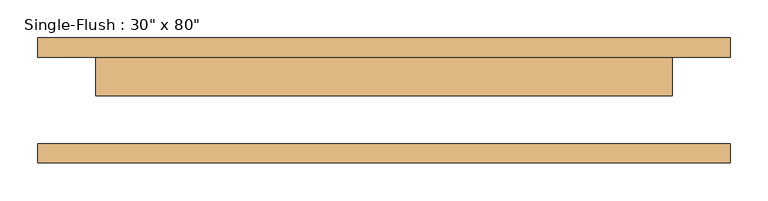
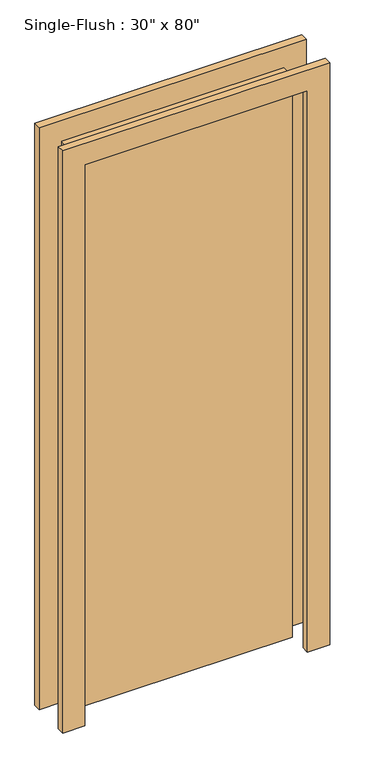
"""IFC4 building model written with IfcOpenShell, lengths in millimetres: door geometry."""

from ifc_helpers import new_model, si_unit, frame, origin, origin_with_axes, place, context, project, spatial, polyline, outline, extrude, source, transform, mapped, element, save


def door_d8f5dbb5(model_context):
    return source(origin(), model_context, "Body", "SweptSolid", [
        extrude(outline(polyline([(2108.2, -457.2), (0.0, -457.2), (0.0, -381.0), (2032.0, -381.0), (2032.0, 381.0), (0.0, 381.0), (0.0, 457.2), (2108.2, 457.2), (2108.2, -457.2)])), frame((0.0, 57.15, 0.0), z_axis=(0.0, 1.0, 0.0), x_axis=(0.0, 0.0, 1.0)), (0.0, 0.0, 1.0), 25.4),
        extrude(outline(polyline([(2108.2, 457.2), (2108.2, -457.2), (0.0, -457.2), (0.0, -381.0), (2032.0, -381.0), (2032.0, 381.0), (0.0, 381.0), (0.0, 457.2), (2108.2, 457.2)])), frame((0.0, -82.55, 0.0), z_axis=(0.0, 1.0, 0.0), x_axis=(0.0, 0.0, 1.0)), (0.0, 0.0, 1.0), 25.4),
        extrude(outline(polyline([(381.0, 6.35), (-381.0, 6.35), (-381.0, 57.15), (381.0, 57.15), (381.0, 6.35)])), origin_with_axes(), (0.0, 0.0, 1.0), 2032.0),
    ])


if __name__ == "__main__":
    model = new_model("IFC4")
    model_context = context("Model", 3, world=origin())
    ifc_project = project(units=[si_unit("LENGTHUNIT", "METRE", prefix="MILLI")], contexts=[model_context])
    site = spatial("IfcSite", under=ifc_project)
    building = spatial("IfcBuilding", under=site)
    placement = place(None, origin())
    door_shape = door_d8f5dbb5(model_context)
    element("IfcDoor", 1, ObjectType="Single-Flush : 30\" x 80\"", at=placement, inside=building, context=model_context, shape_type="MappedRepresentation", body=[
        mapped(door_shape, transform((0.0, 0.0, 0.0), x_axis=(1.0, 0.0, 0.0), y_axis=(0.0, 1.0, 0.0), z_axis=(0.0, 0.0, 1.0))),
    ])
    save(model, "model.ifc")

# Revit data of these elements
# Type "Single-Flush : 30\" x 80\""
#   Type Mark = "5"
#   Construction Type Id = "MDOOR"
#   Assembly Code = "C1020"
#   Analytic Construction = "Metal"
#   Thickness = 0' - 2"
#   Heat Transfer Coefficient (U) = 0.651978 BTU/(h·ft²·°F)
#   Height = 6' - 8"
#   Trim Projection Ext = 0' - 1"
#   Trim Projection Int = 0' - 1"
#   Trim Width = 0' - 3"
#   Width = 2' - 6"
#   Define Thermal Properties by = 1
#   Define Thermal Properties by = 1
#   Door Material = Door - Panel
#   Frame Material = Door - Frame
#   Visual Light Transmittance = 0
#   Solar Heat Gain Coefficient = 0
#   Function = (empty or 0)
#   Wall Closure = (empty or 0)
# Element 1 (IfcDoor, "Single-Flush : 30\" x 80\"")
#   Materials on its faces: "Door - Frame", "Door - Panel"
# Materials
#   "Door - Panel": class "Wood", colour RGB 210 159 95, transparency 0, Cost = 0
#   "Door - Frame": colour RGB 118 70 51, transparency 0, Cost = 0
